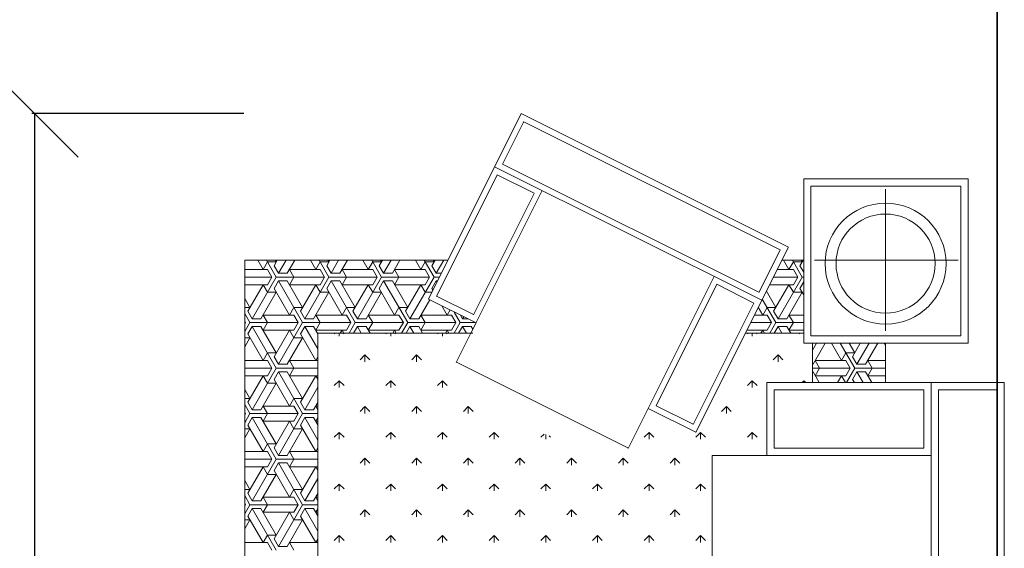
# Model space of a CAD drawing. Units: inches. Extents: x -1198 to -69, y -512 to 437.
# Tile 46 of 50: x -444 to -376, y 77 to 113. Entities that reach past the tile are written whole.
import ezdxf

# ---------------------------------------------------------------- set-up
doc = ezdxf.new("R2010")
doc.units = ezdxf.units.IN
doc.header["$MEASUREMENT"] = 0
for name, color, linetype, lineweight in [('A-ANNO-DIMS', 2, 'Continuous', 18), ('A-FURN', 60, 'Continuous', 18), ('A-WALL', 7, 'Continuous', 35)]:
    doc.layers.add(name, color=color, linetype=linetype, lineweight=lineweight)
doc.styles.get("Standard").update_dxf_attribs({"font": 'arial.ttf'})
doc.dimstyles.get("Standard").update_dxf_attribs({"dimtxt": 6, "dimasz": 6, "dimexe": 0.18, "dimexo": 0.0625, "dimgap": 0.09, "dimtad": 0, "dimtih": 1, "dimtoh": 1, "dimdec": 0, "dimzin": 0, "dimdsep": 46, "dimlunit": 4, "dimtxsty": 'Standard', "dimblk": 'OBLIQUE', "dimcen": 0.09, "dimadec": 0, "dimazin": 0, "dimtfac": 1, "dimtdec": 0, "dimtofl": 0, "dimtmove": 0, "dimatfit": 3, "dimfxl": 1, "dimtolj": 1, "dimtzin": 0, "dimarcsym": 0})

# ---------------------------------------------------------------- blocks, each defined once
blk = doc.blocks.new('A$C3B9F700E')
for p, q in [((736.9, 2080, -685.7), (2936.9, 2080, -685.7)), ((736.9, 2080, -685.7), (736.9, 1430, -685.7)), ((736.9, 1880, -685.7), (736.9, 2080, -685.7)), ((756.9, 2060, -685.7), (2916.9, 2060, -685.7)), ((756.9, 1900, -685.7), (756.9, 2060, -685.7)), ((179, 1980.6, -685.7), (179, 1530.6, -685.7)), ((629, 1980.6, -685.7), (179, 1980.6, -685.7)), ((629, 1530.6, -685.7), (629, 1980.6, -685.7)), ((199, 1960.6, -685.7), (199, 1550.6, -685.7)), ((609, 1960.6, -685.7), (199, 1960.6, -685.7)), ((401.3, 1953.9, -685.7), (401.3, 1560.5, -685.7)), ((609, 1550.6, -685.7), (609, 1960.6, -685.7)), ((2916.9, 1900, -685.7), (756.9, 1900, -685.7)), ((2936.9, 1880, -685.7), (736.9, 1880, -685.7)), ((2936.9, 1880, -685.7), (736.9, 1880, -685.7)), ((736.9, 1430, -685.7), (736.9, 1880, -685.7)), ((736.9, 1880, -685.7), (936.9, 1880, -685.7)), ((936.9, 1880, -685.7), (936.9, 1280, -685.7)), ((936.9, 1880, -685.7), (936.9, 1430, -685.7)), ((756.9, 1450, -685.7), (756.9, 1860, -685.7)), ((756.9, 1860, -685.7), (916.9, 1860, -685.7)), ((916.9, 1860, -685.7), (916.9, 1450, -685.7)), ((595.4, 1754.8, -685.7), (207.1, 1754.8, -685.7)), ((629, 1754.8, -685.7), (736.9, 1754.8, -685.7)), ((629, 1754.8, -685.7), (736.9, 1754.8, -685.7)), ((629, 1554.8, -685.7), (629, 1754.8, -685.7)), ((629, 1750.9, -685.7), (635.7, 1754.8, -685.7)), ((676.4, 1754.8, -685.7), (676.4, 1706.3, -685.7)), ((697.2, 1670.3, -685.7), (697.2, 1754.8, -685.7)), ((718, 1754.8, -685.7), (718, 1706.3, -685.7)), ((736.9, 1754.8, -685.7), (736.9, 1554.8, -685.7)), ((686.8, 1700.3, -685.7), (629, 1733.7, -685.7)), ((629, 1709.7, -685.7), (686.8, 1676.3, -685.7)), ((697.2, 1718.3, -685.7), (676.4, 1706.3, -685.7)), ((686.8, 1676.3, -685.7), (686.8, 1700.3, -685.7)), ((697.2, 1718.3, -685.7), (718, 1706.3, -685.7)), ((707.6, 1700.3, -685.7), (736.9, 1717.3, -685.7)), ((707.6, 1676.3, -685.7), (707.6, 1700.3, -685.7)), ((666, 1664.3, -685.7), (629, 1685.7, -685.7)), ((686.8, 1676.3, -685.7), (666, 1664.3, -685.7)), ((736.9, 1693.3, -685.7), (707.6, 1676.3, -685.7)), ((707.6, 1676.3, -685.7), (728.4, 1664.3, -685.7)), ((629, 1654.9, -685.7), (655.6, 1670.3, -685.7)), ((697.2, 1670.3, -685.7), (629, 1630.9, -685.7)), ((655.6, 1646.3, -685.7), (655.6, 1670.3, -685.7)), ((655.6, 1646.3, -685.7), (676.4, 1634.3, -685.7)), ((697.2, 1658.3, -685.7), (676.4, 1646.3, -685.7)), ((676.4, 1646.3, -685.7), (676.4, 1562.3, -685.7)), ((697.2, 1670.3, -685.7), (736.9, 1647.4, -685.7)), ((697.2, 1658.3, -685.7), (718, 1646.3, -685.7)), ((697.2, 1554.8, -685.7), (697.2, 1658.3, -685.7)), ((718, 1646.3, -685.7), (718, 1562.3, -685.7)), ((736.9, 1645.3, -685.7), (718, 1634.3, -685.7)), ((728.4, 1664.3, -685.7), (736.9, 1669.3, -685.7)), ((629, 1606.9, -685.7), (676.4, 1634.3, -685.7)), ((736.9, 1623.4, -685.7), (718, 1634.3, -685.7)), ((686.8, 1556.3, -685.7), (629, 1589.7, -685.7)), ((629, 1565.7, -685.7), (647.9, 1554.8, -685.7)), ((697.2, 1574.3, -685.7), (676.4, 1562.3, -685.7)), ((697.2, 1574.3, -685.7), (718, 1562.3, -685.7)), ((707.6, 1556.3, -685.7), (736.9, 1573.3, -685.7)), ((199, 1550.6, -685.7), (609, 1550.6, -685.7)), ((736.9, 1554.8, -685.7), (629, 1554.8, -685.7)), ((629, 1554.8, -685.7), (736.9, 1554.8, -685.7)), ((686.8, 1554.8, -685.7), (686.8, 1556.3, -685.7)), ((707.6, 1554.8, -685.7), (707.6, 1556.3, -685.7)), ((179, 1530.6, -685.7), (629, 1530.6, -685.7)), ((401.4, 1530.6, -685.7), (401.4, 1470.6, -685.7)), ((401.4, 1470.6, -685.7), (401.4, 1530.6, -685.7)), ((601.4, 1530.6, -685.7), (401.4, 1530.6, -685.7)), ((416.6, 1520.3, -685.7), (401.4, 1529.1, -685.7)), ((401.4, 1523.6, -685.7), (406.2, 1526.3, -685.7)), ((447.8, 1526.3, -685.7), (401.4, 1499.6, -685.7)), ((406.2, 1502.3, -685.7), (406.2, 1526.3, -685.7)), ((434.4, 1530.6, -685.7), (416.6, 1520.3, -685.7)), ((447.8, 1514.3, -685.7), (427, 1502.3, -685.7)), ((447.8, 1526.3, -685.7), (447.8, 1530.6, -685.7)), ((447.8, 1526.3, -685.7), (562.1, 1460.3, -685.7)), ((447.8, 1514.3, -685.7), (468.6, 1502.3, -685.7)), ((447.8, 1447.5, -685.7), (447.8, 1514.3, -685.7)), ((461.1, 1530.6, -685.7), (479, 1520.3, -685.7)), ((479, 1520.3, -685.7), (496.8, 1530.6, -685.7)), ((562.1, 1484.3, -685.7), (489.3, 1526.3, -685.7)), ((489.3, 1502.3, -685.7), (489.3, 1526.3, -685.7)), ((551.7, 1530.6, -685.7), (551.7, 1490.3, -685.7)), ((572.5, 1454.3, -685.7), (572.5, 1530.6, -685.7)), ((593.3, 1530.6, -685.7), (593.3, 1490.3, -685.7)), ((601.4, 1370.8, -685.7), (601.4, 1530.6, -685.7)), ((601.4, 1370.8, -685.7), (601.4, 1530.6, -685.7)), ((601.4, 1520.3, -685.7), (603.7, 1518, -685.7)), ((731.9, 1531.3, -685.7), (736.9, 1536.3, -685.7)), ((731.9, 1531.3, -685.7), (736.9, 1526.2, -685.7)), ((731.9, 1531.3, -685.7), (736.9, 1531.3, -685.7)), ((365.5, 1488.6, -685.7), (0, 756.7, -685.7)), ((873.7, 1234.8, -685.7), (366.4, 1488.1, -685.7)), ((401.4, 1475.6, -685.7), (427, 1490.3, -685.7)), ((406.2, 1502.3, -685.7), (427, 1490.3, -685.7)), ((427, 1502.3, -685.7), (427, 1457.9, -685.7)), ((468.6, 1502.3, -685.7), (468.6, 1437.1, -685.7)), ((489.3, 1502.3, -685.7), (468.6, 1490.3, -685.7)), ((541.3, 1448.3, -685.7), (468.6, 1490.3, -685.7)), ((572.5, 1502.3, -685.7), (551.7, 1490.3, -685.7)), ((562.1, 1460.3, -685.7), (562.1, 1484.3, -685.7)), ((572.5, 1502.3, -685.7), (593.3, 1490.3, -685.7)), ((582.9, 1484.3, -685.7), (601.4, 1495, -685.7)), ((582.9, 1460.3, -685.7), (582.9, 1484.3, -685.7)), ((373.6, 1466.4, -685.7), (22.8, 763.8, -685.7)), ((489.2, 1408.7, -685.7), (373.6, 1466.4, -685.7)), ((401.4, 1470.6, -685.7), (601.4, 1370.8, -685.7)), ((562.1, 1460.3, -685.7), (541.3, 1448.3, -685.7)), ((601.4, 1471, -685.7), (582.9, 1460.3, -685.7)), ((582.9, 1460.3, -685.7), (601.4, 1449.6, -685.7)), ((661.2, 1460.6, -685.7), (674.4, 1473.8, -685.7)), ((661.2, 1460.6, -685.7), (674.4, 1447.3, -685.7)), ((661.2, 1460.6, -685.7), (679.9, 1460.6, -685.7)), ((486, 1428.4, -685.7), (530.9, 1454.3, -685.7)), ((572.5, 1454.3, -685.7), (508.3, 1417.3, -685.7)), ((530.9, 1430.3, -685.7), (530.9, 1454.3, -685.7)), ((530.9, 1430.3, -685.7), (551.7, 1418.3, -685.7)), ((572.5, 1442.3, -685.7), (551.7, 1430.3, -685.7)), ((551.7, 1430.3, -685.7), (551.7, 1395.6, -685.7)), ((572.5, 1454.3, -685.7), (601.4, 1437.6, -685.7)), ((572.5, 1385.2, -685.7), (572.5, 1442.3, -685.7)), ((572.5, 1442.3, -685.7), (593.3, 1430.3, -685.7)), ((593.3, 1430.3, -685.7), (593.3, 1374.8, -685.7)), ((936.9, 1430, -685.7), (736.9, 1430, -685.7)), ((916.9, 1450, -685.7), (756.9, 1450, -685.7)), ((138.8, 705.9, -685.7), (489.4, 1408.1, -685.7)), ((511.3, 1415.8, -685.7), (145.8, 683.8, -685.7)), ((489.4, 1408.1, -685.7), (489.2, 1408.7, -685.7)), ((530.6, 1406.1, -685.7), (551.7, 1418.3, -685.7)), ((601.4, 1423, -685.7), (593.3, 1418.3, -685.7)), ((601.4, 1413.6, -685.7), (593.3, 1418.3, -685.7)), ((601.4, 1400.9, -685.7), (603.7, 1403.1, -685.7)), ((731.9, 1389.9, -685.7), (745.1, 1403.1, -685.7)), ((873.3, 1389.9, -685.7), (886.5, 1403.1, -685.7)), ((518.9, 1393.8, -685.7), (467.6, 1293.2, -685.7)), ((851.6, 1227.8, -685.7), (518.9, 1393.8, -685.7)), ((601.4, 1389.9, -685.7), (609.2, 1389.9, -685.7)), ((601.4, 1378.9, -685.7), (603.7, 1376.6, -685.7)), ((731.9, 1389.9, -685.7), (750.6, 1389.9, -685.7)), ((731.9, 1389.9, -685.7), (745.1, 1376.6, -685.7)), ((873.3, 1389.9, -685.7), (892, 1389.9, -685.7)), ((873.3, 1389.9, -685.7), (886.5, 1376.6, -685.7)), ((802.6, 1319.2, -685.7), (815.8, 1332.4, -685.7)), ((802.6, 1319.2, -685.7), (815.8, 1305.9, -685.7)), ((802.6, 1319.2, -685.7), (821.3, 1319.2, -685.7)), ((917.2, 1050.1, -685.7), (446.2, 1285.3, -685.7)), ((800.5, 1126.9, -685.7), (467.6, 1293.2, -685.7)), ((2736.9, 1280, -685.7), (936.9, 1280, -685.7)), ((873.3, 1248.4, -685.7), (886.5, 1261.7, -685.7)), ((873.3, 1248.4, -685.7), (886.5, 1235.2, -685.7)), ((873.3, 1248.4, -685.7), (892, 1248.4, -685.7)), ((1014.7, 1248.4, -685.7), (1028, 1261.7, -685.7)), ((1014.7, 1248.4, -685.7), (1028, 1235.2, -685.7)), ((1014.7, 1248.4, -685.7), (1033.5, 1248.4, -685.7)), ((1156.1, 1248.4, -685.7), (1169.4, 1261.7, -685.7)), ((1156.1, 1248.4, -685.7), (1169.4, 1235.2, -685.7)), ((1156.1, 1248.4, -685.7), (1174.9, 1248.4, -685.7)), ((850.8, 1227.7, -685.7), (800.5, 1126.9, -685.7)), ((872.8, 1235.3, -685.7), (807.6, 1104.8, -685.7)), ((944, 1177.7, -685.7), (957.3, 1191, -685.7)), ((1085.4, 1177.7, -685.7), (1098.7, 1191, -685.7)), ((944, 1177.7, -685.7), (957.3, 1164.5, -685.7)), ((944, 1177.7, -685.7), (962.7, 1177.7, -685.7)), ((1085.4, 1177.7, -685.7), (1098.7, 1164.5, -685.7)), ((1085.4, 1177.7, -685.7), (1104.2, 1177.7, -685.7)), ((873.3, 1107, -685.7), (886.5, 1120.3, -685.7)), ((873.3, 1107, -685.7), (886.5, 1093.8, -685.7)), ((873.3, 1107, -685.7), (892, 1107, -685.7)), ((1014.7, 1107, -685.7), (1028, 1120.3, -685.7)), ((1014.7, 1107, -685.7), (1028, 1093.8, -685.7)), ((1014.7, 1107, -685.7), (1033.5, 1107, -685.7)), ((1156.1, 1107, -685.7), (1169.4, 1120.3, -685.7)), ((1156.1, 1107, -685.7), (1169.4, 1093.8, -685.7)), ((1156.1, 1107, -685.7), (1174.9, 1107, -685.7)), ((916.3, 1050.6, -685.7), (681.1, 579.5, -685.7)), ((944, 1036.3, -685.7), (957.3, 1049.6, -685.7)), ((944, 1036.3, -685.7), (957.3, 1023.1, -685.7)), ((944, 1036.3, -685.7), (962.7, 1036.3, -685.7)), ((1085.4, 1036.3, -685.7), (1098.7, 1049.6, -685.7)), ((1085.4, 1036.3, -685.7), (1098.7, 1023.1, -685.7)), ((1085.4, 1036.3, -685.7), (1104.2, 1036.3, -685.7)), ((1014.7, 965.6, -685.7), (1028, 978.9, -685.7)), ((1156.1, 965.6, -685.7), (1169.4, 978.9, -685.7)), ((1014.7, 965.6, -685.7), (1028, 952.3, -685.7)), ((1014.7, 965.6, -685.7), (1033.5, 965.6, -685.7)), ((1156.1, 965.6, -685.7), (1169.4, 952.3, -685.7)), ((1156.1, 965.6, -685.7), (1174.9, 965.6, -685.7)), ((944, 894.9, -685.7), (957.3, 908.1, -685.7)), ((944, 894.9, -685.7), (957.3, 881.6, -685.7)), ((944, 894.9, -685.7), (962.7, 894.9, -685.7)), ((1085.4, 894.9, -685.7), (1098.7, 908.1, -685.7)), ((1085.4, 894.9, -685.7), (1098.7, 881.6, -685.7)), ((1085.4, 894.9, -685.7), (1104.2, 894.9, -685.7)), ((882.6, 833.5, -685.7), (886.5, 837.4, -685.7)), ((1014.7, 824.2, -685.7), (1028, 837.4, -685.7)), ((1156.1, 824.2, -685.7), (1169.4, 837.4, -685.7)), ((682, 579.1, -685.7), (211, 814.3, -685.7)), ((877.8, 819.7, -685.7), (886.5, 810.9, -685.7)), ((879.4, 824.2, -685.7), (892, 824.2, -685.7)), ((1014.7, 824.2, -685.7), (1028, 810.9, -685.7)), ((1014.7, 824.2, -685.7), (1033.5, 824.2, -685.7)), ((1156.1, 824.2, -685.7), (1169.4, 810.9, -685.7)), ((1156.1, 824.2, -685.7), (1174.9, 824.2, -685.7)), ((218.1, 792.2, -685.7), (167.8, 691.5, -685.7)), ((551.2, 626.3, -685.7), (218.6, 792.4, -685.7)), ((508.2, 502.9, -685.7), (0, 756.7, -685.7)), ((22.8, 763.8, -685.7), (23, 763.3, -685.7)), ((23, 763.3, -685.7), (138.2, 705.7, -685.7)), ((944, 753.5, -685.7), (957.3, 766.7, -685.7)), ((1085.4, 753.5, -685.7), (1098.7, 766.7, -685.7)), ((944, 753.5, -685.7), (957.3, 740.2, -685.7)), ((944, 753.5, -685.7), (962.7, 753.5, -685.7)), ((1085.4, 753.5, -685.7), (1098.7, 740.2, -685.7)), ((1085.4, 753.5, -685.7), (1104.2, 753.5, -685.7)), ((138.2, 705.7, -685.7), (138.8, 705.9, -685.7)), ((500.6, 524.8, -685.7), (167.9, 690.9, -685.7)), ((873.3, 682.8, -685.7), (886.5, 696, -685.7)), ((873.3, 682.8, -685.7), (886.5, 669.5, -685.7)), ((873.3, 682.8, -685.7), (892, 682.8, -685.7)), ((1014.7, 682.8, -685.7), (1028, 696, -685.7)), ((1014.7, 682.8, -685.7), (1028, 669.5, -685.7)), ((1014.7, 682.8, -685.7), (1033.5, 682.8, -685.7)), ((1156.1, 682.8, -685.7), (1169.4, 696, -685.7)), ((1156.1, 682.8, -685.7), (1169.4, 669.5, -685.7)), ((1156.1, 682.8, -685.7), (1174.9, 682.8, -685.7)), ((550.5, 626.2, -685.7), (500.2, 525.5, -685.7)), ((573.3, 633.3, -685.7), (508.2, 502.9, -685.7)), ((573.3, 633.3, -685.7), (508.2, 502.9, -685.7)), ((572.5, 590.3, -685.7), (572.5, 631.7, -685.7)), ((601.4, 619.3, -685.7), (573.3, 633.3, -685.7)), ((582.9, 620.3, -685.7), (590.5, 624.7, -685.7)), ((582.9, 596.3, -685.7), (582.9, 620.3, -685.7)), ((601.4, 200, -685.7), (601.4, 624.9, -685.7)), ((802.6, 612, -685.7), (815.8, 625.3, -685.7)), ((944, 612, -685.7), (957.3, 625.3, -685.7)), ((1085.4, 612, -685.7), (1098.7, 625.3, -685.7)), ((562.1, 596.3, -685.7), (551.9, 590.4, -685.7)), ((556.5, 599.6, -685.7), (562.1, 596.3, -685.7)), ((562.1, 596.3, -685.7), (562.1, 610.8, -685.7)), ((601.4, 607, -685.7), (582.9, 596.3, -685.7)), ((582.9, 596.3, -685.7), (601.4, 585.6, -685.7)), ((601.4, 200, -685.7), (601.4, 619.3, -685.7)), ((802.6, 612, -685.7), (815.8, 598.8, -685.7)), ((802.6, 612, -685.7), (821.3, 612, -685.7)), ((944, 612, -685.7), (957.3, 598.8, -685.7)), ((944, 612, -685.7), (962.7, 612, -685.7)), ((1085.4, 612, -685.7), (1098.7, 598.8, -685.7)), ((1085.4, 612, -685.7), (1104.2, 612, -685.7)), ((572.5, 590.3, -685.7), (543.5, 573.6, -685.7)), ((572.5, 578.3, -685.7), (551.7, 566.3, -685.7)), ((551.7, 566.3, -685.7), (551.7, 482.3, -685.7)), ((572.5, 590.3, -685.7), (601.4, 573.6, -685.7)), ((572.5, 578.3, -685.7), (593.3, 566.3, -685.7)), ((572.5, 446.3, -685.7), (572.5, 578.3, -685.7)), ((593.3, 566.3, -685.7), (593.3, 482.3, -685.7)), ((401.4, 556.2, -685.7), (401.4, 0, -685.7)), ((508.2, 502.9, -685.7), (401.4, 556.2, -685.7)), ((401.4, 0, -685.7), (401.4, 556.2, -685.7)), ((401.4, 545.1, -685.7), (437.4, 524.3, -685.7)), ((526.6, 539.9, -685.7), (551.7, 554.3, -685.7)), ((537.9, 562.3, -685.7), (551.7, 554.3, -685.7)), ((601.4, 559, -685.7), (593.3, 554.3, -685.7)), ((601.4, 549.6, -685.7), (593.3, 554.3, -685.7)), ((601.4, 552.3, -685.7), (603.7, 554.6, -685.7)), ((601.4, 541.3, -685.7), (609.2, 541.3, -685.7)), ((731.9, 541.3, -685.7), (745.1, 554.6, -685.7)), ((731.9, 541.3, -685.7), (745.1, 528.1, -685.7)), ((731.9, 541.3, -685.7), (750.6, 541.3, -685.7)), ((873.3, 541.3, -685.7), (886.5, 554.6, -685.7)), ((873.3, 541.3, -685.7), (886.5, 528.1, -685.7)), ((873.3, 541.3, -685.7), (892, 541.3, -685.7)), ((1014.7, 541.3, -685.7), (1028, 554.6, -685.7)), ((1014.7, 541.3, -685.7), (1028, 528.1, -685.7)), ((1014.7, 541.3, -685.7), (1033.5, 541.3, -685.7)), ((1156.1, 541.3, -685.7), (1169.4, 554.6, -685.7)), ((1156.1, 541.3, -685.7), (1169.4, 528.1, -685.7)), ((1156.1, 541.3, -685.7), (1174.9, 541.3, -685.7)), ((416.6, 512.3, -685.7), (401.4, 521.1, -685.7)), ((401.4, 515.6, -685.7), (406.2, 518.3, -685.7)), ((447.8, 518.3, -685.7), (401.4, 491.6, -685.7)), ((406.2, 494.3, -685.7), (406.2, 518.3, -685.7)), ((437.4, 524.3, -685.7), (416.6, 512.3, -685.7)), ((437.4, 524.3, -685.7), (437.4, 538.3, -685.7)), ((447.8, 518.3, -685.7), (447.8, 533.1, -685.7)), ((447.8, 518.3, -685.7), (562.1, 452.3, -685.7)), ((458.2, 524.3, -685.7), (458.2, 527.9, -685.7)), ((461.5, 526.2, -685.7), (458.2, 524.3, -685.7)), ((458.2, 524.3, -685.7), (479, 512.3, -685.7)), ((479, 512.3, -685.7), (483.8, 515.1, -685.7)), ((489.3, 494.3, -685.7), (489.3, 512.3, -685.7)), ((601.4, 530.3, -685.7), (603.7, 528.1, -685.7)), ((406.2, 494.3, -685.7), (427, 482.3, -685.7)), ((447.8, 506.3, -685.7), (427, 494.3, -685.7)), ((427, 494.3, -685.7), (427, 410.3, -685.7)), ((447.8, 506.3, -685.7), (468.6, 494.3, -685.7)), ((447.8, 374.3, -685.7), (447.8, 506.3, -685.7)), ((468.6, 494.3, -685.7), (468.6, 410.3, -685.7)), ((489.3, 494.3, -685.7), (468.6, 482.3, -685.7)), ((562.1, 476.3, -685.7), (509.9, 506.4, -685.7)), ((572.5, 494.3, -685.7), (551.7, 482.3, -685.7)), ((572.5, 494.3, -685.7), (593.3, 482.3, -685.7)), ((582.9, 476.3, -685.7), (601.4, 487, -685.7)), ((401.4, 467.6, -685.7), (427, 482.3, -685.7)), ((541.3, 440.3, -685.7), (468.6, 482.3, -685.7)), ((562.1, 452.3, -685.7), (562.1, 476.3, -685.7)), ((582.9, 452.3, -685.7), (582.9, 476.3, -685.7)), ((601.4, 463, -685.7), (582.9, 452.3, -685.7)), ((661.2, 470.6, -685.7), (674.4, 483.9, -685.7)), ((661.2, 470.6, -685.7), (679.9, 470.6, -685.7)), ((661.2, 470.6, -685.7), (674.4, 457.4, -685.7)), ((802.6, 470.6, -685.7), (815.8, 483.9, -685.7)), ((802.6, 470.6, -685.7), (821.3, 470.6, -685.7)), ((802.6, 470.6, -685.7), (815.8, 457.4, -685.7)), ((944, 470.6, -685.7), (957.3, 483.9, -685.7)), ((944, 470.6, -685.7), (962.7, 470.6, -685.7)), ((944, 470.6, -685.7), (957.3, 457.4, -685.7)), ((1085.4, 470.6, -685.7), (1098.7, 483.9, -685.7)), ((1085.4, 470.6, -685.7), (1104.2, 470.6, -685.7)), ((1085.4, 470.6, -685.7), (1098.7, 457.4, -685.7)), ((458.2, 404.3, -685.7), (530.9, 446.3, -685.7)), ((572.5, 446.3, -685.7), (458.2, 380.3, -685.7)), ((530.9, 422.3, -685.7), (530.9, 446.3, -685.7)), ((562.1, 452.3, -685.7), (541.3, 440.3, -685.7)), ((572.5, 434.3, -685.7), (551.7, 422.3, -685.7)), ((572.5, 446.3, -685.7), (601.4, 429.6, -685.7)), ((572.5, 434.3, -685.7), (593.3, 422.3, -685.7)), ((572.5, 302.3, -685.7), (572.5, 434.3, -685.7)), ((582.9, 452.3, -685.7), (601.4, 441.6, -685.7)), ((437.4, 404.3, -685.7), (401.4, 425.1, -685.7)), ((447.8, 422.3, -685.7), (427, 410.3, -685.7)), ((447.8, 422.3, -685.7), (468.6, 410.3, -685.7)), ((479, 368.3, -685.7), (551.7, 410.3, -685.7)), ((530.9, 422.3, -685.7), (551.7, 410.3, -685.7)), ((551.7, 422.3, -685.7), (551.7, 338.3, -685.7)), ((593.3, 422.3, -685.7), (593.3, 338.3, -685.7)), ((601.4, 415, -685.7), (593.3, 410.3, -685.7)), ((601.4, 405.6, -685.7), (593.3, 410.3, -685.7)), ((601.4, 410.9, -685.7), (603.7, 413.2, -685.7)), ((731.9, 399.9, -685.7), (745.1, 413.2, -685.7)), ((873.3, 399.9, -685.7), (886.5, 413.2, -685.7)), ((1014.7, 399.9, -685.7), (1028, 413.2, -685.7)), ((1156.1, 399.9, -685.7), (1169.4, 413.2, -685.7)), ((401.4, 401.1, -685.7), (437.4, 380.3, -685.7)), ((437.4, 380.3, -685.7), (416.6, 368.3, -685.7)), ((437.4, 380.3, -685.7), (437.4, 404.3, -685.7)), ((458.2, 380.3, -685.7), (458.2, 404.3, -685.7)), ((458.2, 380.3, -685.7), (479, 368.3, -685.7)), ((601.4, 399.9, -685.7), (609.2, 399.9, -685.7)), ((601.4, 388.9, -685.7), (603.7, 386.7, -685.7)), ((731.9, 399.9, -685.7), (750.6, 399.9, -685.7)), ((731.9, 399.9, -685.7), (745.1, 386.7, -685.7)), ((873.3, 399.9, -685.7), (892, 399.9, -685.7)), ((873.3, 399.9, -685.7), (886.5, 386.7, -685.7)), ((1014.7, 399.9, -685.7), (1033.5, 399.9, -685.7)), ((1014.7, 399.9, -685.7), (1028, 386.7, -685.7)), ((1156.1, 399.9, -685.7), (1174.9, 399.9, -685.7)), ((1156.1, 399.9, -685.7), (1169.4, 386.7, -685.7)), ((416.6, 368.3, -685.7), (401.4, 377.1, -685.7)), ((401.4, 371.6, -685.7), (406.2, 374.3, -685.7)), ((447.8, 374.3, -685.7), (401.4, 347.6, -685.7)), ((406.2, 350.3, -685.7), (406.2, 374.3, -685.7)), ((447.8, 362.3, -685.7), (427, 350.3, -685.7)), ((447.8, 374.3, -685.7), (562.1, 308.3, -685.7)), ((447.8, 362.3, -685.7), (468.6, 350.3, -685.7)), ((447.8, 230.3, -685.7), (447.8, 362.3, -685.7)), ((562.1, 332.3, -685.7), (489.3, 374.3, -685.7)), ((489.3, 350.3, -685.7), (489.3, 374.3, -685.7)), ((401.4, 323.6, -685.7), (427, 338.3, -685.7)), ((406.2, 350.3, -685.7), (427, 338.3, -685.7)), ((427, 350.3, -685.7), (427, 266.3, -685.7)), ((468.6, 350.3, -685.7), (468.6, 266.3, -685.7)), ((489.3, 350.3, -685.7), (468.6, 338.3, -685.7)), ((541.3, 296.3, -685.7), (468.6, 338.3, -685.7)), ((572.5, 350.3, -685.7), (551.7, 338.3, -685.7)), ((562.1, 308.3, -685.7), (562.1, 332.3, -685.7)), ((572.5, 350.3, -685.7), (593.3, 338.3, -685.7)), ((582.9, 332.3, -685.7), (601.4, 343, -685.7)), ((582.9, 308.3, -685.7), (582.9, 332.3, -685.7)), ((661.2, 329.2, -685.7), (674.4, 342.5, -685.7)), ((661.2, 329.2, -685.7), (674.4, 315.9, -685.7)), ((661.2, 329.2, -685.7), (679.9, 329.2, -685.7)), ((802.6, 329.2, -685.7), (815.8, 342.5, -685.7)), ((802.6, 329.2, -685.7), (815.8, 315.9, -685.7)), ((802.6, 329.2, -685.7), (821.3, 329.2, -685.7)), ((944, 329.2, -685.7), (957.3, 342.5, -685.7)), ((944, 329.2, -685.7), (957.3, 315.9, -685.7)), ((944, 329.2, -685.7), (962.7, 329.2, -685.7)), ((1085.4, 329.2, -685.7), (1098.7, 342.5, -685.7)), ((1085.4, 329.2, -685.7), (1098.7, 315.9, -685.7)), ((1085.4, 329.2, -685.7), (1104.2, 329.2, -685.7)), ((458.2, 260.3, -685.7), (530.9, 302.3, -685.7)), ((572.5, 302.3, -685.7), (458.2, 236.3, -685.7)), ((530.9, 278.3, -685.7), (530.9, 302.3, -685.7)), ((562.1, 308.3, -685.7), (541.3, 296.3, -685.7)), ((572.5, 302.3, -685.7), (601.4, 285.6, -685.7)), ((601.4, 319, -685.7), (582.9, 308.3, -685.7)), ((582.9, 308.3, -685.7), (601.4, 297.6, -685.7)), ((437.4, 260.3, -685.7), (401.4, 281.1, -685.7)), ((447.8, 278.3, -685.7), (427, 266.3, -685.7)), ((447.8, 278.3, -685.7), (468.6, 266.3, -685.7)), ((530.9, 278.3, -685.7), (551.7, 266.3, -685.7)), ((572.5, 290.3, -685.7), (551.7, 278.3, -685.7)), ((551.7, 278.3, -685.7), (551.7, 194.3, -685.7)), ((572.5, 290.3, -685.7), (593.3, 278.3, -685.7)), ((572.5, 158.3, -685.7), (572.5, 290.3, -685.7)), ((593.3, 278.3, -685.7), (593.3, 194.3, -685.7)), ((601.4, 271, -685.7), (593.3, 266.3, -685.7)), ((601.4, 269.5, -685.7), (603.7, 271.8, -685.7)), ((731.9, 258.5, -685.7), (745.1, 271.8, -685.7)), ((873.3, 258.5, -685.7), (886.5, 271.8, -685.7)), ((1014.7, 258.5, -685.7), (1028, 271.8, -685.7)), ((1156.1, 258.5, -685.7), (1169.4, 271.8, -685.7)), ((401.4, 257.1, -685.7), (437.4, 236.3, -685.7)), ((437.4, 236.3, -685.7), (437.4, 260.3, -685.7)), ((458.2, 236.3, -685.7), (458.2, 260.3, -685.7)), ((479, 224.3, -685.7), (551.7, 266.3, -685.7)), ((601.4, 261.6, -685.7), (593.3, 266.3, -685.7)), ((601.4, 258.5, -685.7), (609.2, 258.5, -685.7)), ((601.4, 247.5, -685.7), (603.7, 245.2, -685.7)), ((731.9, 258.5, -685.7), (745.1, 245.2, -685.7)), ((731.9, 258.5, -685.7), (750.6, 258.5, -685.7)), ((873.3, 258.5, -685.7), (886.5, 245.2, -685.7)), ((873.3, 258.5, -685.7), (892, 258.5, -685.7)), ((1014.7, 258.5, -685.7), (1028, 245.2, -685.7)), ((1014.7, 258.5, -685.7), (1033.5, 258.5, -685.7)), ((1156.1, 258.5, -685.7), (1169.4, 245.2, -685.7)), ((1156.1, 258.5, -685.7), (1174.9, 258.5, -685.7)), ((416.6, 224.3, -685.7), (401.4, 233.1, -685.7)), ((401.4, 227.6, -685.7), (406.2, 230.3, -685.7)), ((447.8, 230.3, -685.7), (401.4, 203.6, -685.7)), ((406.2, 206.3, -685.7), (406.2, 230.3, -685.7)), ((437.4, 236.3, -685.7), (416.6, 224.3, -685.7)), ((447.8, 218.3, -685.7), (427, 206.3, -685.7)), ((447.8, 230.3, -685.7), (562.1, 164.3, -685.7)), ((447.8, 218.3, -685.7), (468.6, 206.3, -685.7)), ((447.8, 86.3, -685.7), (447.8, 218.3, -685.7)), ((458.2, 236.3, -685.7), (479, 224.3, -685.7)), ((562.1, 188.3, -685.7), (489.3, 230.3, -685.7)), ((489.3, 206.3, -685.7), (489.3, 230.3, -685.7)), ((401.4, 179.6, -685.7), (427, 194.3, -685.7)), ((406.2, 206.3, -685.7), (427, 194.3, -685.7)), ((427, 206.3, -685.7), (427, 122.3, -685.7)), ((468.6, 206.3, -685.7), (468.6, 122.3, -685.7)), ((489.3, 206.3, -685.7), (468.6, 194.3, -685.7)), ((541.3, 152.3, -685.7), (468.6, 194.3, -685.7)), ((572.5, 206.3, -685.7), (551.7, 194.3, -685.7)), ((572.5, 206.3, -685.7), (593.3, 194.3, -685.7)), ((582.9, 188.3, -685.7), (603.1, 200, -685.7)), ((644.7, 200, -685.7), (582.9, 164.3, -685.7)), ((3062.1, 200, -685.7), (601.4, 200, -685.7)), ((3062.1, 200, -685.7), (601.4, 200, -685.7)), ((603.7, 152.3, -685.7), (676.4, 194.3, -685.7)), ((666.6, 200, -685.7), (676.4, 194.3, -685.7)), ((673.4, 200, -685.7), (674.4, 201, -685.7)), ((676.4, 200, -685.7), (676.4, 122.3, -685.7)), ((697.2, 86.3, -685.7), (697.2, 200, -685.7)), ((718, 200, -685.7), (718, 122.3, -685.7)), ((727.8, 200, -685.7), (718, 194.3, -685.7)), ((790.7, 152.3, -685.7), (718, 194.3, -685.7)), ((749.7, 200, -685.7), (811.5, 164.3, -685.7)), ((811.5, 188.3, -685.7), (791.3, 200, -685.7)), ((801.1, 200, -685.7), (801.1, 194.3, -685.7)), ((811, 200, -685.7), (801.1, 194.3, -685.7)), ((814.8, 200, -685.7), (815.8, 201, -685.7)), ((821.9, 158.3, -685.7), (821.9, 200, -685.7)), ((832.3, 188.3, -685.7), (852.5, 200, -685.7)), ((894.1, 200, -685.7), (832.3, 164.3, -685.7)), ((832.8, 200, -685.7), (842.7, 194.3, -685.7)), ((842.7, 200, -685.7), (842.7, 194.3, -685.7)), ((853.1, 152.3, -685.7), (925.8, 194.3, -685.7)), ((916, 200, -685.7), (925.8, 194.3, -685.7)), ((925.8, 200, -685.7), (925.8, 122.3, -685.7)), ((946.6, 86.3, -685.7), (946.6, 200, -685.7)), ((956.2, 200, -685.7), (957.3, 201, -685.7)), ((967.4, 200, -685.7), (967.4, 122.3, -685.7)), ((977.2, 200, -685.7), (967.4, 194.3, -685.7)), ((1040.1, 152.3, -685.7), (967.4, 194.3, -685.7)), ((999.1, 200, -685.7), (1060.9, 164.3, -685.7)), ((1060.9, 188.3, -685.7), (1040.7, 200, -685.7)), ((1050.5, 200, -685.7), (1050.5, 194.3, -685.7)), ((1060.4, 200, -685.7), (1050.5, 194.3, -685.7)), ((1071.3, 158.3, -685.7), (1071.3, 200, -685.7)), ((1081.7, 188.3, -685.7), (1101.9, 200, -685.7)), ((1143.5, 200, -685.7), (1081.7, 164.3, -685.7)), ((1082.3, 200, -685.7), (1092.1, 194.3, -685.7)), ((1092.1, 200, -685.7), (1092.1, 194.3, -685.7)), ((1097.6, 200, -685.7), (1098.7, 201, -685.7)), ((1102.5, 152.3, -685.7), (1175.2, 194.3, -685.7)), ((1165.4, 200, -685.7), (1175.2, 194.3, -685.7)), ((1175.2, 200, -685.7), (1175.2, 122.3, -685.7)), ((562.1, 164.3, -685.7), (541.3, 152.3, -685.7)), ((562.1, 164.3, -685.7), (562.1, 188.3, -685.7)), ((582.9, 164.3, -685.7), (582.9, 188.3, -685.7)), ((582.9, 164.3, -685.7), (603.7, 152.3, -685.7)), ((811.5, 164.3, -685.7), (790.7, 152.3, -685.7)), ((811.5, 164.3, -685.7), (811.5, 188.3, -685.7)), ((832.3, 164.3, -685.7), (832.3, 188.3, -685.7)), ((832.3, 164.3, -685.7), (853.1, 152.3, -685.7)), ((1060.9, 164.3, -685.7), (1040.1, 152.3, -685.7)), ((1060.9, 164.3, -685.7), (1060.9, 188.3, -685.7)), ((1081.7, 164.3, -685.7), (1081.7, 188.3, -685.7)), ((1081.7, 164.3, -685.7), (1102.5, 152.3, -685.7)), ((437.4, 116.3, -685.7), (401.4, 137.1, -685.7)), ((458.2, 116.3, -685.7), (530.9, 158.3, -685.7)), ((572.5, 158.3, -685.7), (458.2, 92.3, -685.7)), ((530.9, 134.3, -685.7), (530.9, 158.3, -685.7)), ((572.5, 146.3, -685.7), (551.7, 134.3, -685.7)), ((572.5, 158.3, -685.7), (686.8, 92.3, -685.7)), ((572.5, 146.3, -685.7), (593.3, 134.3, -685.7)), ((572.5, 14.3, -685.7), (572.5, 146.3, -685.7)), ((686.8, 116.3, -685.7), (614.1, 158.3, -685.7)), ((614.1, 134.3, -685.7), (614.1, 158.3, -685.7)), ((707.6, 116.3, -685.7), (780.3, 158.3, -685.7)), ((821.9, 158.3, -685.7), (707.6, 92.3, -685.7)), ((780.3, 134.3, -685.7), (780.3, 158.3, -685.7)), ((821.9, 146.3, -685.7), (801.1, 134.3, -685.7)), ((821.9, 158.3, -685.7), (936.2, 92.3, -685.7)), ((821.9, 146.3, -685.7), (842.7, 134.3, -685.7)), ((821.9, 14.3, -685.7), (821.9, 146.3, -685.7)), ((936.2, 116.3, -685.7), (863.5, 158.3, -685.7)), ((863.5, 134.3, -685.7), (863.5, 158.3, -685.7)), ((957, 116.3, -685.7), (1029.7, 158.3, -685.7)), ((1071.3, 158.3, -685.7), (957, 92.3, -685.7)), ((1029.7, 134.3, -685.7), (1029.7, 158.3, -685.7)), ((1071.3, 146.3, -685.7), (1050.5, 134.3, -685.7)), ((1071.3, 158.3, -685.7), (1185.6, 92.3, -685.7)), ((1071.3, 146.3, -685.7), (1092.1, 134.3, -685.7)), ((1071.3, 14.3, -685.7), (1071.3, 146.3, -685.7)), ((1185.6, 116.3, -685.7), (1112.9, 158.3, -685.7)), ((1112.9, 134.3, -685.7), (1112.9, 158.3, -685.7)), ((401.4, 113.1, -685.7), (437.4, 92.3, -685.7)), ((447.8, 134.3, -685.7), (427, 122.3, -685.7)), ((437.4, 92.3, -685.7), (437.4, 116.3, -685.7)), ((447.8, 134.3, -685.7), (468.6, 122.3, -685.7)), ((458.2, 92.3, -685.7), (458.2, 116.3, -685.7)), ((479, 80.3, -685.7), (551.7, 122.3, -685.7)), ((530.9, 134.3, -685.7), (551.7, 122.3, -685.7)), ((551.7, 134.3, -685.7), (551.7, 50.3, -685.7)), ((593.3, 134.3, -685.7), (593.3, 50.3, -685.7)), ((614.1, 134.3, -685.7), (593.3, 122.3, -685.7)), ((666, 80.3, -685.7), (593.3, 122.3, -685.7)), ((697.2, 134.3, -685.7), (676.4, 122.3, -685.7)), ((686.8, 92.3, -685.7), (686.8, 116.3, -685.7)), ((697.2, 134.3, -685.7), (718, 122.3, -685.7)), ((707.6, 92.3, -685.7), (707.6, 116.3, -685.7)), ((728.4, 80.3, -685.7), (801.1, 122.3, -685.7)), ((780.3, 134.3, -685.7), (801.1, 122.3, -685.7)), ((801.1, 134.3, -685.7), (801.1, 50.3, -685.7)), ((842.7, 134.3, -685.7), (842.7, 50.3, -685.7)), ((863.5, 134.3, -685.7), (842.7, 122.3, -685.7)), ((915.4, 80.3, -685.7), (842.7, 122.3, -685.7)), ((946.6, 134.3, -685.7), (925.8, 122.3, -685.7)), ((936.2, 92.3, -685.7), (936.2, 116.3, -685.7)), ((946.6, 134.3, -685.7), (967.4, 122.3, -685.7)), ((957, 92.3, -685.7), (957, 116.3, -685.7)), ((977.8, 80.3, -685.7), (1050.5, 122.3, -685.7)), ((1029.7, 134.3, -685.7), (1050.5, 122.3, -685.7)), ((1050.5, 134.3, -685.7), (1050.5, 50.3, -685.7)), ((1092.1, 134.3, -685.7), (1092.1, 50.3, -685.7)), ((1112.9, 134.3, -685.7), (1092.1, 122.3, -685.7)), ((1164.8, 80.3, -685.7), (1092.1, 122.3, -685.7)), ((1196, 134.3, -685.7), (1175.2, 122.3, -685.7)), ((1185.6, 92.3, -685.7), (1185.6, 116.3, -685.7)), ((416.6, 80.3, -685.7), (401.4, 89.1, -685.7)), ((401.4, 83.6, -685.7), (406.2, 86.3, -685.7)), ((447.8, 86.3, -685.7), (401.4, 59.6, -685.7)), ((406.2, 62.3, -685.7), (406.2, 86.3, -685.7)), ((437.4, 92.3, -685.7), (416.6, 80.3, -685.7)), ((447.8, 86.3, -685.7), (562.1, 20.3, -685.7)), ((458.2, 92.3, -685.7), (479, 80.3, -685.7)), ((562.1, 44.3, -685.7), (489.3, 86.3, -685.7)), ((489.3, 62.3, -685.7), (489.3, 86.3, -685.7)), ((582.9, 44.3, -685.7), (655.6, 86.3, -685.7)), ((697.2, 86.3, -685.7), (582.9, 20.3, -685.7)), ((655.6, 62.3, -685.7), (655.6, 86.3, -685.7)), ((686.8, 92.3, -685.7), (666, 80.3, -685.7)), ((697.2, 86.3, -685.7), (811.5, 20.3, -685.7)), ((707.6, 92.3, -685.7), (728.4, 80.3, -685.7)), ((811.5, 44.3, -685.7), (738.8, 86.3, -685.7)), ((738.8, 62.3, -685.7), (738.8, 86.3, -685.7)), ((832.3, 44.3, -685.7), (905, 86.3, -685.7)), ((946.6, 86.3, -685.7), (832.3, 20.3, -685.7)), ((905, 62.3, -685.7), (905, 86.3, -685.7)), ((936.2, 92.3, -685.7), (915.4, 80.3, -685.7)), ((946.6, 86.3, -685.7), (1060.9, 20.3, -685.7)), ((957, 92.3, -685.7), (977.8, 80.3, -685.7)), ((988.2, 62.3, -685.7), (988.2, 86.3, -685.7)), ((1060.9, 44.3, -685.7), (988.2, 86.3, -685.7)), ((1081.7, 44.3, -685.7), (1154.5, 86.3, -685.7)), ((1196, 86.3, -685.7), (1081.7, 20.3, -685.7)), ((1154.5, 62.3, -685.7), (1154.5, 86.3, -685.7)), ((1185.6, 92.3, -685.7), (1164.8, 80.3, -685.7)), ((406.2, 62.3, -685.7), (427, 50.3, -685.7)), ((447.8, 74.3, -685.7), (427, 62.3, -685.7)), ((427, 62.3, -685.7), (427, 0, -685.7)), ((447.8, 74.3, -685.7), (468.6, 62.3, -685.7)), ((447.8, 0, -685.7), (447.8, 74.3, -685.7)), ((468.6, 62.3, -685.7), (468.6, 0, -685.7)), ((489.3, 62.3, -685.7), (468.6, 50.3, -685.7)), ((572.5, 62.3, -685.7), (551.7, 50.3, -685.7)), ((572.5, 62.3, -685.7), (593.3, 50.3, -685.7)), ((655.6, 62.3, -685.7), (676.4, 50.3, -685.7)), ((697.2, 74.3, -685.7), (676.4, 62.3, -685.7)), ((676.4, 62.3, -685.7), (676.4, 0, -685.7)), ((697.2, 74.3, -685.7), (718, 62.3, -685.7)), ((697.2, 0, -685.7), (697.2, 74.3, -685.7)), ((718, 62.3, -685.7), (718, 0, -685.7)), ((738.8, 62.3, -685.7), (718, 50.3, -685.7)), ((821.9, 62.3, -685.7), (801.1, 50.3, -685.7)), ((821.9, 62.3, -685.7), (842.7, 50.3, -685.7)), ((905, 62.3, -685.7), (925.8, 50.3, -685.7)), ((946.6, 74.3, -685.7), (925.8, 62.3, -685.7)), ((925.8, 62.3, -685.7), (925.8, 0, -685.7)), ((946.6, 74.3, -685.7), (967.4, 62.3, -685.7)), ((946.6, 0, -685.7), (946.6, 74.3, -685.7)), ((967.4, 62.3, -685.7), (967.4, 0, -685.7)), ((988.2, 62.3, -685.7), (967.4, 50.3, -685.7)), ((1071.3, 62.3, -685.7), (1050.5, 50.3, -685.7)), ((1071.3, 62.3, -685.7), (1092.1, 50.3, -685.7)), ((1154.5, 62.3, -685.7), (1175.2, 50.3, -685.7)), ((1196, 74.3, -685.7), (1175.2, 62.3, -685.7)), ((1175.2, 62.3, -685.7), (1175.2, 0, -685.7)), ((401.4, 35.6, -685.7), (427, 50.3, -685.7)), ((541.3, 8.3, -685.7), (468.6, 50.3, -685.7)), ((562.1, 20.3, -685.7), (562.1, 44.3, -685.7)), ((582.9, 20.3, -685.7), (582.9, 44.3, -685.7)), ((603.7, 8.3, -685.7), (676.4, 50.3, -685.7)), ((790.7, 8.3, -685.7), (718, 50.3, -685.7)), ((811.5, 20.3, -685.7), (811.5, 44.3, -685.7)), ((832.3, 20.3, -685.7), (832.3, 44.3, -685.7)), ((853.1, 8.3, -685.7), (925.8, 50.3, -685.7)), ((1040.1, 8.3, -685.7), (967.4, 50.3, -685.7)), ((1060.9, 20.3, -685.7), (1060.9, 44.3, -685.7)), ((1081.7, 20.3, -685.7), (1081.7, 44.3, -685.7)), ((1102.5, 8.3, -685.7), (1175.2, 50.3, -685.7)), ((401.4, 0, -685.7), (3262.1, 0, -685.7)), ((3262.1, 0, -685.7), (401.4, 0, -685.7)), ((506.1, 0, -685.7), (530.9, 14.3, -685.7)), ((530.9, 0, -685.7), (530.9, 14.3, -685.7)), ((562.1, 20.3, -685.7), (541.3, 8.3, -685.7)), ((572.5, 14.3, -685.7), (547.7, 0, -685.7)), ((572.5, 2.3, -685.7), (568.5, 0, -685.7)), ((572.5, 14.3, -685.7), (597.3, 0, -685.7)), ((572.5, 2.3, -685.7), (576.5, 0, -685.7)), ((572.5, 0, -685.7), (572.5, 2.3, -685.7)), ((582.9, 20.3, -685.7), (603.7, 8.3, -685.7)), ((638.9, 0, -685.7), (614.1, 14.3, -685.7)), ((614.1, 0, -685.7), (614.1, 14.3, -685.7)), ((755.5, 0, -685.7), (780.3, 14.3, -685.7)), ((780.3, 0, -685.7), (780.3, 14.3, -685.7)), ((811.5, 20.3, -685.7), (790.7, 8.3, -685.7)), ((821.9, 14.3, -685.7), (797.1, 0, -685.7)), ((821.9, 2.3, -685.7), (817.9, 0, -685.7)), ((821.9, 14.3, -685.7), (846.7, 0, -685.7)), ((821.9, 2.3, -685.7), (825.9, 0, -685.7)), ((821.9, 0, -685.7), (821.9, 2.3, -685.7)), ((832.3, 20.3, -685.7), (853.1, 8.3, -685.7)), ((888.3, 0, -685.7), (863.5, 14.3, -685.7)), ((863.5, 0, -685.7), (863.5, 14.3, -685.7)), ((1004.9, 0, -685.7), (1029.7, 14.3, -685.7)), ((1029.7, 0, -685.7), (1029.7, 14.3, -685.7)), ((1060.9, 20.3, -685.7), (1040.1, 8.3, -685.7)), ((1071.3, 14.3, -685.7), (1046.5, 0, -685.7)), ((1071.3, 2.3, -685.7), (1067.3, 0, -685.7)), ((1071.3, 14.3, -685.7), (1096.1, 0, -685.7)), ((1071.3, 2.3, -685.7), (1075.3, 0, -685.7)), ((1071.3, 0, -685.7), (1071.3, 2.3, -685.7)), ((1081.7, 20.3, -685.7), (1102.5, 8.3, -685.7)), ((1137.7, 0, -685.7), (1112.9, 14.3, -685.7)), ((1112.9, 0, -685.7), (1112.9, 14.3, -685.7))]:
    blk.add_line(p, q)
for radius in [165.7, 135.7]:
    blk.add_circle((410.9, 1754.8, -685.7), radius)
blk = doc.blocks.new('1')
blk.add_blockref('A$C3B9F700E', (-1861.1, 172.7, 685.7))
blk = doc.blocks.new('_Oblique')
at = {"color": 0, "linetype": 'ByBlock', "lineweight": -2}
blk.add_line((-0.5, -0.5), (0.5, 0.5), dxfattribs=at)
blk = doc.blocks.new('*D52')
at = {"layer": 'A-ANNO-DIMS', "color": 0, "lineweight": -2, "ltscale": 10, "transparency": 16777216}
for p, q in [((-428.646, 106.551), (-443.249, 106.551)), ((-443.069, 106.551), (-443.069, 61.46)), ((-443.069, 9.981), (-443.069, 55.072)), ((-428.646, 9.981), (-443.249, 9.981))]:
    blk.add_line(p, q, dxfattribs=at)
at = {"layer": 'DEFPOINTS', "color": 0, "ltscale": 10, "transparency": 16777216}
for p in [(-428.584, 106.551), (-443.069, 9.981), (-428.584, 9.981)]:
    blk.add_point(p, dxfattribs=at)
at = {"layer": 'A-ANNO-DIMS', "color": 0, "lineweight": -2, "ltscale": 10, "transparency": 16777216, "xscale": 6, "yscale": 6, "zscale": 6}
for p, rotation in [((-443.069, 106.551), 90), ((-443.069, 9.981), 270)]:
    blk.add_blockref('_Oblique', p, dxfattribs=dict(at, rotation=rotation))
at = {"layer": 'A-ANNO-DIMS', "color": 0, "ltscale": 10, "transparency": 16777216, "insert": (-443.069, 58.266), "char_height": 6, "attachment_point": 5}
blk.add_mtext('\\A1;SEATING GROUP 97 TYP.', dxfattribs=at)

msp = doc.modelspace()

# ---------------------------------------------------------------- linework, layer by layer
at = {"layer": 'A-WALL', "ltscale": 10}
msp.add_line((-376.7509, -222.7723), (-376.7509, 257.2277), dxfattribs=at)

# ---------------------------------------------------------------- block references
at = {"layer": 'A-FURN', "ltscale": 10, "xscale": 0.0251614738227896, "yscale": 0.0251614738227896, "zscale": 0.0251614738227896, "rotation": 270.0000000000001}
msp.add_blockref('1', (-432.9284, 59.7223), dxfattribs=at)

# ---------------------------------------------------------------- dimensions: what is measured, and where the dimension line sits
at = {"layer": 'A-ANNO-DIMS', "ltscale": 10}
dim = msp.add_linear_dim(base=(-443.0692, 9.981), p1=(-428.5837, 106.551), p2=(-428.5837, 9.981), angle=270, text='SEATING GROUP <> TYP.', dimstyle='Standard', override={"dimdec": 0, "dimlfac": 1, "dimrnd": 0, "dimzin": 0, "dimdsep": 46, "dimlunit": 2}, dxfattribs=at)
dim.commit()
dim.dimension.update_dxf_attribs({"geometry": '*D52', "text_midpoint": (-443.0692, 58.266)})

doc.saveas('drawing.dxf')
